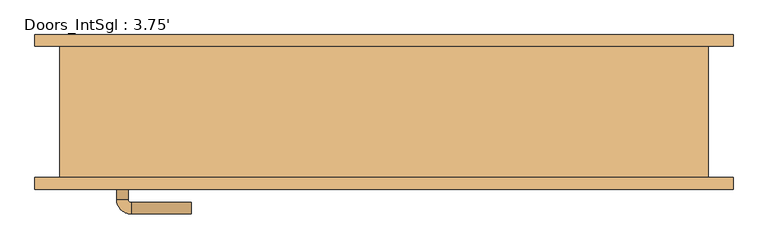
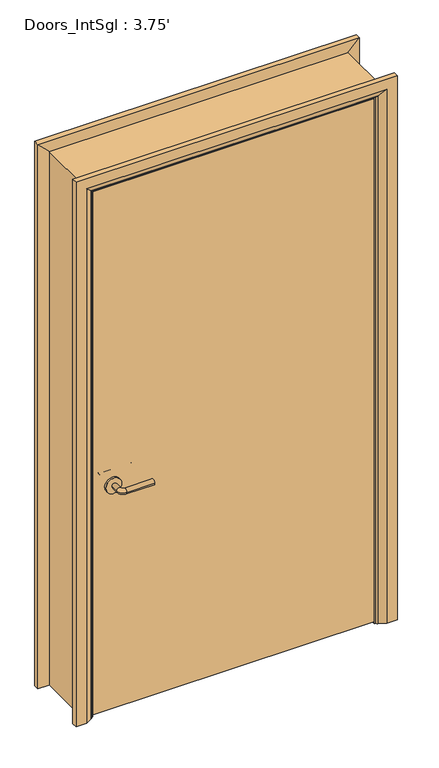
"""IFC4 building model written with IfcOpenShell, lengths in millimetres: door geometry, Doors_IntSgl : 3.75'."""

from ifc_helpers import new_model, si_unit, point, frame, frame_2d, origin, place, context, project, spatial, polyline, circle_curve, ellipse_curve, trimmed, segment, composite_curve, outline, extrude, faceted_brep, source, transform, mapped, element, save
from ifc_brep_helpers import plane_surface, cylinder_surface, revolved_surface, advanced_brep


def doors_intsgl_3_75_7d887cbf(model_context):
    return source(origin(), model_context, "Body", "SolidModel", [
        advanced_brep(
        [(-464.5, -68.3, 900.0), (-444.5, -68.3, 900.0), (-464.5, -38.3, 900.0), (-444.5, -38.3, 900.0), (-439.5, -33.3, 900.0), (-439.5, -13.3, 900.0), (-334.5, -13.3, 900.0), (-334.5, -33.3, 900.0)],
        [
            (0, 1, circle_curve(frame((-454.5, -68.3, 900.0), z_axis=(0.0, -1.0, 0.0), x_axis=(1.0, 0.0, 0.0)), 10.0)),
            (1, 0, circle_curve(frame((-454.5, -68.3, 900.0), z_axis=(0.0, -1.0, 0.0), x_axis=(1.0, 0.0, 0.0)), 10.0)),
            (0, 2),
            (2, 3, circle_curve(frame((-454.5, -38.3, 900.0), z_axis=(0.0, -1.0, 0.0), x_axis=(1.0, 0.0, 0.0)), 10.0)),
            (3, 1),
            (3, 2, circle_curve(frame((-454.5, -38.3, 900.0), z_axis=(0.0, -1.0, 0.0), x_axis=(1.0, 0.0, 0.0)), 10.0)),
            (4, 3, circle_curve(frame((-439.5, -38.3, 900.0), z_axis=(0.0, 0.0, 1.0), x_axis=(-1.0, 0.0, 0.0)), 5.0)),
            (2, 5, circle_curve(frame((-439.5, -38.3, 900.0), z_axis=(0.0, 0.0, -1.0), x_axis=(-1.0, 0.0, 0.0)), 25.0)),
            (5, 4, circle_curve(frame((-439.5, -23.3, 900.0), z_axis=(-1.0, 0.0, 0.0), x_axis=(0.0, -1.0, 0.0)), 10.0)),
            (4, 5, circle_curve(frame((-439.5, -23.3, 900.0), z_axis=(-1.0, 0.0, 0.0), x_axis=(0.0, -1.0, 0.0)), 10.0)),
            (6, 7, circle_curve(frame((-334.5, -23.3, 900.0), z_axis=(1.0, 0.0, 0.0), x_axis=(0.0, -1.0, 0.0)), 10.0)),
            (7, 6, circle_curve(frame((-334.5, -23.3, 900.0), z_axis=(1.0, 0.0, 0.0), x_axis=(0.0, -1.0, 0.0)), 10.0)),
            (5, 6),
            (7, 4),
        ],
        [
            plane_surface(frame((-454.5, -68.3, 900.0), z_axis=(0.0, -1.0, 0.0), x_axis=(0.0, 0.0, 1.0))),
            cylinder_surface(frame((-454.5, -68.3, 900.0), z_axis=(0.0, -1.0, 0.0), x_axis=(1.0, 0.0, 0.0)), 10.0),
            revolved_surface(trimmed(ellipse_curve(frame((-454.5, -38.3, 900.0), z_axis=(0.0, -1.0, 0.0), x_axis=(1.0, 0.0, 0.0)), 10.0, 10.0), [point((-464.5, -38.3, 900.0))], [point((-444.5, -38.3, 900.0))], True, "CARTESIAN"), (-439.5, -38.3, 900.0), (0.0, 0.0, -1.0)),
            revolved_surface(trimmed(ellipse_curve(frame((-454.5, -38.3, 900.0), z_axis=(0.0, -1.0, 0.0), x_axis=(1.0, 0.0, 0.0)), 10.0, 10.0), [point((-444.5, -38.3, 900.0))], [point((-464.5, -38.3, 900.0))], True, "CARTESIAN"), (-439.5, -38.3, 900.0), (0.0, 0.0, -1.0)),
            plane_surface(frame((-334.5, -23.3, 900.0), z_axis=(1.0, 0.0, 0.0), x_axis=(0.0, 0.0, 1.0))),
            cylinder_surface(frame((-439.5, -23.3, 900.0), z_axis=(-1.0, 0.0, 0.0), x_axis=(0.0, -1.0, 0.0)), 10.0),
        ],
        [
            (0, [[1, 2]]),
            (1, [[-1, 3, 4, 5]]),
            (1, [[-2, -5, 6, -3]]),
            (2, [[7, -4, 8, 9]]),
            (3, [[-8, -6, -7, 10]]),
            (4, [[11, 12]]),
            (5, [[-9, 13, -12, 14]]),
            (5, [[-10, -14, -11, -13]]),
        ],
    ),
        extrude(outline(composite_curve([segment(trimmed(circle_curve(frame_2d((900.0, -457.0)), 30.0), [point((900.0, -487.0))], [point((900.0, -427.0))], False, "CARTESIAN"), True, "CONTINUOUS"), segment(trimmed(circle_curve(frame_2d((900.0, -457.0)), 30.0), [point((900.0, -427.0))], [point((900.0, -487.0))], False, "CARTESIAN"), True, "CONTINUOUS")], self_intersect=False)), frame((0.0, -76.3, 0.0), z_axis=(0.0, 1.0, 0.0), x_axis=(0.0, 0.0, 1.0)), (0.0, 0.0, 1.0), 8.0),
        advanced_brep(
        [(-464.5, -122.3, 900.0), (-444.5, -122.3, 900.0), (-444.5, -152.3, 900.0), (-464.5, -152.3, 900.0), (-439.5, -157.3, 900.0), (-439.5, -177.3, 900.0), (-334.5, -177.3, 900.0), (-334.5, -157.3, 900.0)],
        [
            (0, 1, circle_curve(frame((-454.5, -122.3, 900.0), z_axis=(0.0, 1.0, 0.0), x_axis=(1.0, 0.0, 0.0)), 10.0)),
            (1, 0, circle_curve(frame((-454.5, -122.3, 900.0), z_axis=(0.0, 1.0, 0.0), x_axis=(1.0, 0.0, 0.0)), 10.0)),
            (1, 2),
            (2, 3, circle_curve(frame((-454.5, -152.3, 900.0), z_axis=(0.0, 1.0, 0.0), x_axis=(1.0, 0.0, 0.0)), 10.0)),
            (3, 0),
            (3, 2, circle_curve(frame((-454.5, -152.3, 900.0), z_axis=(0.0, 1.0, 0.0), x_axis=(1.0, 0.0, 0.0)), 10.0)),
            (4, 5, circle_curve(frame((-439.5, -167.3, 900.0), z_axis=(-1.0, 0.0, 0.0), x_axis=(0.0, 1.0, 0.0)), 10.0)),
            (5, 3, circle_curve(frame((-439.5, -152.3, 900.0), z_axis=(0.0, 0.0, -1.0), x_axis=(-1.0, 0.0, 0.0)), 25.0)),
            (2, 4, circle_curve(frame((-439.5, -152.3, 900.0), z_axis=(0.0, 0.0, 1.0), x_axis=(-1.0, 0.0, 0.0)), 5.0)),
            (5, 4, circle_curve(frame((-439.5, -167.3, 900.0), z_axis=(-1.0, 0.0, 0.0), x_axis=(0.0, 1.0, 0.0)), 10.0)),
            (6, 7, circle_curve(frame((-334.5, -167.3, 900.0), z_axis=(1.0, 0.0, 0.0), x_axis=(0.0, 1.0, 0.0)), 10.0)),
            (7, 6, circle_curve(frame((-334.5, -167.3, 900.0), z_axis=(1.0, 0.0, 0.0), x_axis=(0.0, 1.0, 0.0)), 10.0)),
            (4, 7),
            (6, 5),
        ],
        [
            plane_surface(frame((-454.5, -122.3, 900.0), z_axis=(0.0, 1.0, 0.0), x_axis=(0.0, 0.0, 1.0))),
            cylinder_surface(frame((-454.5, -122.3, 900.0), z_axis=(0.0, 1.0, 0.0), x_axis=(1.0, 0.0, 0.0)), 10.0),
            revolved_surface(trimmed(ellipse_curve(frame((-454.5, -152.3, 900.0), z_axis=(0.0, -1.0, 0.0), x_axis=(1.0, 0.0, 0.0)), 10.0, 10.0), [point((-464.5, -152.3, 900.0))], [point((-444.5, -152.3, 900.0))], True, "CARTESIAN"), (-439.5, -152.3, 900.0), (0.0, 0.0, -1.0)),
            revolved_surface(trimmed(ellipse_curve(frame((-454.5, -152.3, 900.0), z_axis=(0.0, -1.0, 0.0), x_axis=(1.0, 0.0, 0.0)), 10.0, 10.0), [point((-444.5, -152.3, 900.0))], [point((-464.5, -152.3, 900.0))], True, "CARTESIAN"), (-439.5, -152.3, 900.0), (0.0, 0.0, -1.0)),
            plane_surface(frame((-334.5, -167.3, 900.0), z_axis=(1.0, 0.0, 0.0), x_axis=(0.0, 0.0, 1.0))),
            cylinder_surface(frame((-439.5, -167.3, 900.0), z_axis=(-1.0, 0.0, 0.0), x_axis=(0.0, 1.0, 0.0)), 10.0),
        ],
        [
            (0, [[1, 2]]),
            (1, [[3, 4, 5, -2]]),
            (1, [[-5, 6, -3, -1]]),
            (2, [[7, 8, -4, 9]]),
            (3, [[10, -9, -6, -8]]),
            (4, [[11, 12]]),
            (5, [[13, -11, 14, -7]]),
            (5, [[-14, -12, -13, -10]]),
        ],
    ),
        extrude(outline(composite_curve([segment(trimmed(circle_curve(frame_2d((900.0, -457.0)), 30.0), [point((900.0, -487.0))], [point((900.0, -427.0))], False, "CARTESIAN"), True, "CONTINUOUS"), segment(trimmed(circle_curve(frame_2d((900.0, -457.0)), 30.0), [point((900.0, -427.0))], [point((900.0, -487.0))], False, "CARTESIAN"), True, "CONTINUOUS")], self_intersect=False)), frame((0.0, -122.3, 0.0), z_axis=(0.0, 1.0, 0.0), x_axis=(0.0, 0.0, 1.0)), (0.0, 0.0, 1.0), 8.0),
        extrude(outline(polyline([(529.5, -76.3), (529.5, -114.3), (-529.5, -114.3), (-529.5, -76.3), (529.5, -76.3)])), frame((0.0, 0.0, 8.0), z_axis=(0.0, 0.0, 1.0), x_axis=(1.0, 0.0, 0.0)), (0.0, 0.0, 1.0), 2083.6),
        advanced_brep(
        [(606.5, -134.3, 0.0), (566.5, -134.3, 0.0), (540.5, -120.3, 0.0), (536.5, -114.3, 0.0), (606.5, -114.3, 0.0), (606.5, -114.3, 2168.6), (606.5, -134.3, 2168.6), (536.5, -114.3, 2098.6), (-536.5, -114.3, 2098.6), (-536.5, -114.3, 0.0), (-606.5, -114.3, 0.0), (-606.5, -114.3, 2168.6), (540.5, -120.3, 2102.6), (566.5, -134.3, 2128.6), (-606.5, -134.3, 2168.6), (-606.5, -134.3, 0.0), (-566.5, -134.3, 0.0), (-566.5, -134.3, 2128.6), (-540.5, -120.3, 0.0), (-540.5, -120.3, 2102.6)],
        [
            (0, 1),
            (1, 2),
            (2, 3, circle_curve(frame((544.5, -113.3, 0.0), z_axis=(0.0, 0.0, -1.0), x_axis=(1.0, 0.0, 0.0)), 8.0622577)),
            (3, 4),
            (4, 0),
            (4, 5),
            (5, 6),
            (6, 0),
            (3, 7),
            (7, 8),
            (8, 9),
            (9, 10),
            (10, 11),
            (11, 5),
            (2, 12),
            (12, 7, ellipse_curve(frame((544.5, -113.3, 2106.6), z_axis=(0.7071067811865475, 0.0, -0.7071067811865475), x_axis=(-0.7071067811865474, 0.0, -0.7071067811865476)), 11.4017543, 8.0622577)),
            (1, 13),
            (13, 12),
            (6, 14),
            (14, 15),
            (15, 16),
            (16, 17),
            (17, 13),
            (10, 15),
            (14, 11),
            (9, 18, circle_curve(frame((-544.5, -113.3, 0.0), z_axis=(0.0, 0.0, -1.0), x_axis=(-1.0, 0.0, 0.0)), 8.0622577)),
            (18, 16),
            (19, 18),
            (8, 19, ellipse_curve(frame((-544.5, -113.3, 2106.6), z_axis=(-0.7071067811865475, 0.0, -0.7071067811865475), x_axis=(-0.7071067811865474, 0.0, 0.7071067811865476)), 11.4017543, 8.0622577)),
            (19, 17),
            (12, 19),
        ],
        [
            plane_surface(frame((536.5, -114.3, 0.0), z_axis=(0.0, 0.0, -1.0), x_axis=(0.0, 1.0, 0.0))),
            plane_surface(frame((606.5, -134.3, 0.0), z_axis=(1.0, 0.0, 0.0), x_axis=(0.0, 0.0, 1.0))),
            plane_surface(frame((606.5, -114.3, 0.0), z_axis=(0.0, 1.0, 0.0), x_axis=(0.0, 0.0, 1.0))),
            cylinder_surface(frame((544.5, -113.3, 0.0), z_axis=(0.0, 0.0, -1.0), x_axis=(1.0, 0.0, 0.0)), 8.0622577),
            plane_surface(frame((540.5, -120.3, 0.0), z_axis=(-0.4740998230350126, -0.880471099922178, 0.0), x_axis=(0.0, 0.0, 1.0))),
            plane_surface(frame((566.5, -134.3, 0.0), z_axis=(0.0, -1.0, 0.0), x_axis=(0.0, 0.0, 1.0))),
            plane_surface(frame((-606.5, -134.3, 2168.6), z_axis=(-1.0, 0.0, 0.0), x_axis=(0.0, 0.0, -1.0))),
            plane_surface(frame((-536.5, -114.3, 0.0), z_axis=(0.0, 0.0, -1.0), x_axis=(0.0, 1.0, 0.0))),
            cylinder_surface(frame((-544.5, -113.3, 2098.6), z_axis=(0.0, 0.0, 1.0), x_axis=(-1.0, 0.0, 0.0)), 8.0622577),
            plane_surface(frame((-540.5, -120.3, 2102.6), z_axis=(0.47409982303501824, -0.8804710999221749, 0.0), x_axis=(0.0, 0.0, -1.0))),
            plane_surface(frame((606.5, -134.3, 2168.6), z_axis=(0.0, 0.0, 1.0), x_axis=(-1.0, 0.0, 0.0))),
            cylinder_surface(frame((536.5, -113.3, 2106.6), z_axis=(1.0, 0.0, 0.0), x_axis=(0.0, 0.0, 1.0)), 8.0622577),
            plane_surface(frame((540.5, -120.3, 2102.6), z_axis=(0.0, -0.8804710999221764, -0.4740998230350154), x_axis=(-1.0, 0.0, 0.0))),
        ],
        [
            (0, [[1, 2, 3, 4, 5]]),
            (1, [[6, 7, 8, -5]]),
            (2, [[9, 10, 11, 12, 13, 14, -6, -4]]),
            (3, [[15, 16, -9, -3]]),
            (4, [[17, 18, -15, -2]]),
            (5, [[-8, 19, 20, 21, 22, 23, -17, -1]]),
            (6, [[-13, 24, -20, 25]]),
            (7, [[-24, -12, 26, 27, -21]]),
            (8, [[28, -26, -11, 29]]),
            (9, [[-22, -27, -28, 30]]),
            (10, [[-14, -25, -19, -7]]),
            (11, [[31, -29, -10, -16]]),
            (12, [[-23, -30, -31, -18]]),
        ],
    ),
        extrude(outline(polyline([(0.0, -512.5), (2074.6, -512.5), (2074.6, 512.5), (0.0, 512.5), (0.0, 531.5), (2093.6, 531.5), (2093.6, -531.5), (0.0, -531.5), (0.0, -512.5)])), frame((0.0, -74.3, 0.0), z_axis=(0.0, 1.0, 0.0), x_axis=(0.0, 0.0, 1.0)), (0.0, 0.0, 1.0), 32.0),
        advanced_brep(
        [(-606.5, 134.3, 0.0), (-566.5, 134.3, 0.0), (-540.5, 120.3, 0.0), (-536.5, 114.3, 0.0), (-606.5, 114.3, 0.0), (-606.5, 114.3, 2168.6), (-606.5, 134.3, 2168.6), (-536.5, 114.3, 2098.6), (-540.5, 120.3, 2102.6), (-566.5, 134.3, 2128.6), (606.5, 134.3, 0.0), (606.5, 114.3, 0.0), (536.5, 114.3, 0.0), (540.5, 120.3, 0.0), (566.5, 134.3, 0.0), (606.5, 134.3, 2168.6), (566.5, 134.3, 2128.6), (540.5, 120.3, 2102.6), (536.5, 114.3, 2098.6), (606.5, 114.3, 2168.6)],
        [
            (0, 1),
            (1, 2),
            (2, 3, circle_curve(frame((-544.5, 113.3, 0.0), z_axis=(0.0, 0.0, -1.0), x_axis=(-1.0, 0.0, 0.0)), 8.0622577)),
            (3, 4),
            (4, 0),
            (4, 5),
            (5, 6),
            (6, 0),
            (3, 7),
            (7, 5),
            (2, 8),
            (8, 7, ellipse_curve(frame((-544.5, 113.3, 2106.6), z_axis=(-0.7071067811865475, 0.0, -0.7071067811865475), x_axis=(0.7071067811865474, 0.0, -0.7071067811865476)), 11.4017543, 8.0622577)),
            (1, 9),
            (9, 8),
            (6, 9),
            (10, 11),
            (11, 12),
            (12, 13, circle_curve(frame((544.5, 113.3, 0.0), z_axis=(0.0, 0.0, -1.0), x_axis=(1.0, 0.0, 0.0)), 8.0622577)),
            (13, 14),
            (14, 10),
            (15, 10),
            (14, 16),
            (16, 15),
            (13, 17),
            (17, 16),
            (12, 18),
            (18, 17, ellipse_curve(frame((544.5, 113.3, 2106.6), z_axis=(0.7071067811865475, 0.0, -0.7071067811865475), x_axis=(0.7071067811865474, 0.0, 0.7071067811865476)), 11.4017543, 8.0622577)),
            (11, 19),
            (19, 18),
            (15, 19),
            (5, 19),
            (15, 6),
            (7, 18),
            (8, 17),
            (9, 16),
        ],
        [
            plane_surface(frame((-536.5, 187.1010989, 0.0), z_axis=(0.0, 0.0, -1.0), x_axis=(1.0, 0.0, 0.0))),
            plane_surface(frame((-606.5, 134.3, 0.0), z_axis=(-1.0, 0.0, 0.0), x_axis=(0.0, 0.0, 1.0))),
            plane_surface(frame((-606.5, 114.3, 0.0), z_axis=(0.0, -1.0, 0.0), x_axis=(0.0, 0.0, 1.0))),
            cylinder_surface(frame((-544.5, 113.3, 0.0), z_axis=(0.0, 0.0, -1.0), x_axis=(-1.0, 0.0, 0.0)), 8.0622577),
            plane_surface(frame((-540.5, 120.3, 0.0), z_axis=(0.4740998230350183, 0.8804710999221749, 0.0), x_axis=(0.0, 0.0, 1.0))),
            plane_surface(frame((-566.5, 134.3, 0.0), z_axis=(0.0, 1.0, 0.0), x_axis=(0.0, 0.0, 1.0))),
            plane_surface(frame((536.5, 187.1010989, 0.0), z_axis=(0.0, 0.0, -1.0), x_axis=(-1.0, 0.0, 0.0))),
            plane_surface(frame((566.5, 134.3, 2128.6), z_axis=(0.0, 1.0, 0.0), x_axis=(0.0, 0.0, -1.0))),
            plane_surface(frame((540.5, 120.3, 2102.6), z_axis=(-0.4740998230350183, 0.8804710999221749, 0.0), x_axis=(0.0, 0.0, -1.0))),
            cylinder_surface(frame((544.5, 113.3, 2098.6), z_axis=(0.0, 0.0, 1.0), x_axis=(1.0, 0.0, 0.0)), 8.0622577),
            plane_surface(frame((606.5, 114.3, 2168.6), z_axis=(0.0, -1.0, 0.0), x_axis=(0.0, 0.0, -1.0))),
            plane_surface(frame((606.5, 134.3, 2168.6), z_axis=(1.0, 0.0, 0.0), x_axis=(0.0, 0.0, -1.0))),
            plane_surface(frame((-606.5, 134.3, 2168.6), z_axis=(0.0, 0.0, 1.0), x_axis=(1.0, 0.0, 0.0))),
            plane_surface(frame((-606.5, 114.3, 2168.6), z_axis=(0.0, -1.0, 0.0), x_axis=(1.0, 0.0, 0.0))),
            cylinder_surface(frame((-536.5, 113.3, 2106.6), z_axis=(-1.0, 0.0, 0.0), x_axis=(0.0, 0.0, 1.0)), 8.0622577),
            plane_surface(frame((-540.5, 120.3, 2102.6), z_axis=(0.0, 0.8804710999221749, -0.4740998230350183), x_axis=(1.0, 0.0, 0.0))),
            plane_surface(frame((-566.5, 134.3, 2128.6), z_axis=(0.0, 1.0, 0.0), x_axis=(1.0, 0.0, 0.0))),
        ],
        [
            (0, [[1, 2, 3, 4, 5]]),
            (1, [[6, 7, 8, -5]]),
            (2, [[9, 10, -6, -4]]),
            (3, [[11, 12, -9, -3]]),
            (4, [[13, 14, -11, -2]]),
            (5, [[-8, 15, -13, -1]]),
            (6, [[16, 17, 18, 19, 20]]),
            (7, [[21, -20, 22, 23]]),
            (8, [[-22, -19, 24, 25]]),
            (9, [[-24, -18, 26, 27]]),
            (10, [[-26, -17, 28, 29]]),
            (11, [[-28, -16, -21, 30]]),
            (12, [[31, -30, 32, -7]]),
            (13, [[33, -29, -31, -10]]),
            (14, [[34, -27, -33, -12]]),
            (15, [[35, -25, -34, -14]]),
            (16, [[-32, -23, -35, -15]]),
        ],
    ),
        faceted_brep([(-531.5, -114.3, 0.0), (-563.5, -114.3, 0.0), (-563.5, 114.3, 0.0), (-531.5, 114.3, 0.0), (-531.5, 114.3, 2093.6), (-531.5, -114.3, 2093.6), (-563.5, 114.3, 2125.6), (-563.5, -114.3, 2125.6), (531.5, -114.3, 0.0), (531.5, 114.3, 0.0), (563.5, 114.3, 0.0), (563.5, -114.3, 0.0), (531.5, -114.3, 2093.6), (563.5, -114.3, 2125.6), (563.5, 114.3, 2125.6), (531.5, 114.3, 2093.6)], [[[0, 1, 2, 3]], [[3, 4, 5, 0]], [[2, 6, 4, 3]], [[1, 7, 6, 2]], [[0, 5, 7, 1]], [[8, 9, 10, 11]], [[12, 8, 11, 13]], [[13, 11, 10, 14]], [[14, 10, 9, 15]], [[15, 9, 8, 12]], [[4, 15, 12, 5]], [[6, 14, 15, 4]], [[7, 13, 14, 6]], [[5, 12, 13, 7]]]),
    ])


if __name__ == "__main__":
    model = new_model("IFC4")
    model_context = context("Model", 3, world=origin())
    ifc_project = project(units=[si_unit("LENGTHUNIT", "METRE", prefix="MILLI")], contexts=[model_context])
    site = spatial("IfcSite", under=ifc_project)
    building = spatial("IfcBuilding", under=site)
    placement = place(None, origin())
    doors_intsgl_3_75_shape = doors_intsgl_3_75_7d887cbf(model_context)
    element("IfcDoor", 1, ObjectType="Doors_IntSgl : 3.75'", at=placement, inside=building, context=model_context, shape_type="MappedRepresentation", body=[
        mapped(doors_intsgl_3_75_shape, transform((0.0, 0.0, 0.0), x_axis=(1.0, 0.0, 0.0), y_axis=(0.0, 1.0, 0.0), z_axis=(0.0, 0.0, 1.0))),
    ])
    save(model, "model.ifc")

# Revit data of these elements
# Type "Doors_IntSgl : 3.75'"
#   Type Mark = "58"
#   Type Comments = "Internal Single"
#   Operation = "SingleSwingRight"
#   Manufacturer = "Revit"
#   Keynote = "L20"
#   Description = "Internal Single Door"
#   Analytic Construction = "Metal"
#   UnderCut = 8 mm
#   Tolerance = 2 mm
#   Thickness = 38 mm
#   Thermal Resistance (R) = 0.270117 (m²·K)/W
#   Structural Tolerance = 8 mm
#   StopDepth = 32 mm
#   Stop Thickness = 19 mm
#   Rough Width = 1143 mm
#   Rough Height = 2133.6 mm
#   Height to Top Lock Rail = 1000 mm
#   Heat Transfer Coefficient (U) = 3.7021 W/(m²·K)
#   Handle Z Distance = 900 mm
#   Handle X Distance = 75 mm
#   Frame Thickness = 32 mm
#   Door Panel Width = 1059 mm
#   Door Panel Thickness = 38 mm
#   Door Panel Offset = 0 mm
#   Height = 2133.6 mm
#   Width = 1143 mm
#   Door Panel Height = 2083.6 mm
#   Architrave Setback = 5 mm
#   Vis - Ironmongery = yes
#   Material Ironmongery = Door - Handle
#   Material Frame = Door - Frame/Mullion (1)
#   Material Door = Door - Panel
#   Material Architrave = Door - Architrave
#   Visual Light Transmittance = 0
#   Solar Heat Gain Coefficient = 0
#   Function = (empty or 0)
#   Wall Closure = (empty or 0)
# Element 1 (IfcDoor, "Doors_IntSgl : 3.75'")
#   Materials on its faces: "Door - Architrave", "Door - Handle", "Door - Frame/Mullion (1)", "Door - Panel"
# Materials
#   "Door - Handle": colour RGB 0 0 0, transparency 0, Keynote = "P21", Cost = 0
#   "Door - Frame/Mullion (1)": class "Wood", colour RGB 212 179 113, transparency 0, Keynote = "L20", Cost = 0
#   "Door - Panel": class "Wood", colour RGB 210 159 95, transparency 0, Keynote = "L20", Cost = 0
#   "Door - Architrave": class "Wood", colour RGB 154 90 5, transparency 0, Keynote = "P20", Cost = 0
